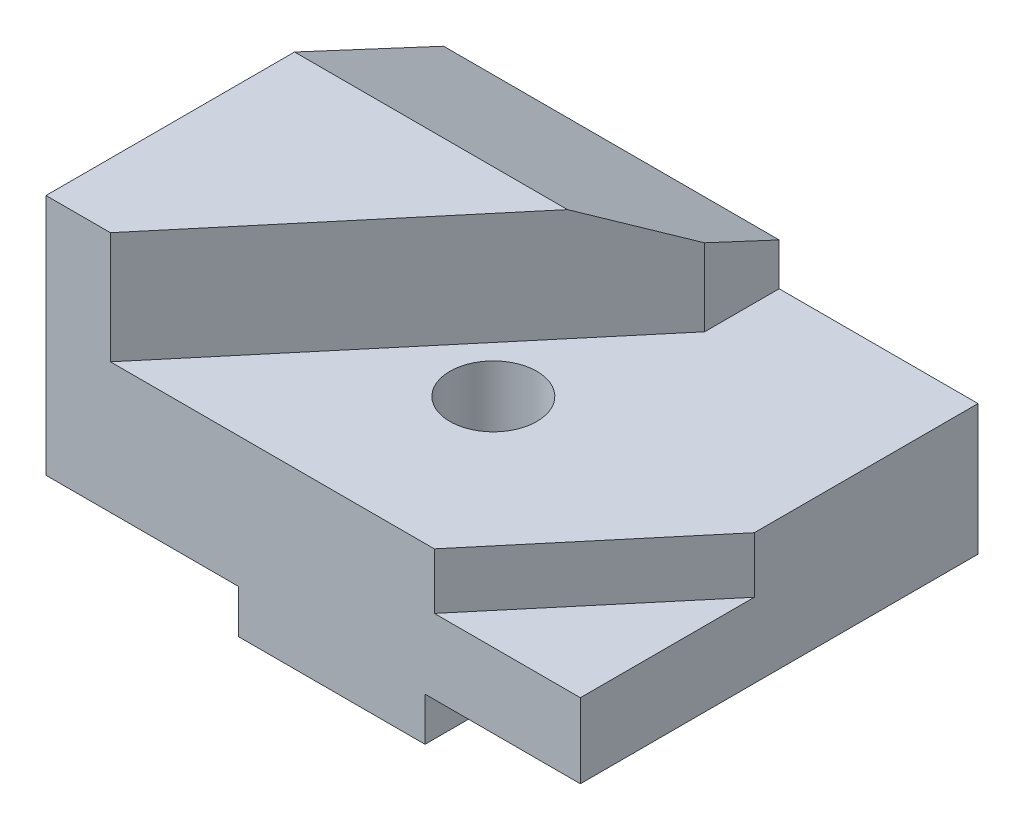
ISO-10303-21;
HEADER;
FILE_DESCRIPTION(('STEP AP214'),'2;1');
FILE_NAME('part.step','',(''),(''),'','','');
FILE_SCHEMA(('AUTOMOTIVE_DESIGN { 1 0 10303 214 1 1 1 1 }'));
ENDSEC;
DATA;
#1=APPLICATION_CONTEXT('core data for automotive mechanical design processes');
#2=APPLICATION_PROTOCOL_DEFINITION('international standard','automotive_design',2000,#1);
#3=PRODUCT_CONTEXT('',#1,'mechanical');
#4=PRODUCT('Part','Part','',(#3));
#5=PRODUCT_RELATED_PRODUCT_CATEGORY('part','',(#4));
#6=PRODUCT_DEFINITION_FORMATION('','',#4);
#7=PRODUCT_DEFINITION_CONTEXT('part definition',#1,'design');
#8=PRODUCT_DEFINITION('design','',#6,#7);
#9=PRODUCT_DEFINITION_SHAPE('','',#8);
#10=(LENGTH_UNIT() NAMED_UNIT(*) SI_UNIT(.MILLI.,.METRE.));
#11=(NAMED_UNIT(*) PLANE_ANGLE_UNIT() SI_UNIT($,.RADIAN.));
#12=(NAMED_UNIT(*) SI_UNIT($,.STERADIAN.) SOLID_ANGLE_UNIT());
#13=UNCERTAINTY_MEASURE_WITH_UNIT(LENGTH_MEASURE(1.E-05),#10,'distance_accuracy_value','');
#14=(GEOMETRIC_REPRESENTATION_CONTEXT(3) GLOBAL_UNCERTAINTY_ASSIGNED_CONTEXT((#13)) GLOBAL_UNIT_ASSIGNED_CONTEXT((#10,
#11,#12)) REPRESENTATION_CONTEXT('',''));
#15=CARTESIAN_POINT('',(0.,0.,0.));
#16=DIRECTION('',(0.,0.,1.));
#17=DIRECTION('',(1.,0.,0.));
#18=AXIS2_PLACEMENT_3D('',#15,#16,#17);
#19=CARTESIAN_POINT('',(0.,0.,0.));
#20=DIRECTION('',(0.,-1.,0.));
#21=DIRECTION('',(0.,0.,-1.));
#22=AXIS2_PLACEMENT_3D('',#19,#20,#21);
#23=PLANE('',#22);
#24=DIRECTION('',(-1.,0.,0.));
#25=VECTOR('',#24,1.);
#26=CARTESIAN_POINT('',(-43.,0.,-32.));
#27=LINE('',#26,#25);
#28=CARTESIAN_POINT('',(-12.,0.,-32.));
#29=VERTEX_POINT('',#28);
#30=CARTESIAN_POINT('',(-43.,0.,-32.));
#31=VERTEX_POINT('',#30);
#32=EDGE_CURVE('E231',#29,#31,#27,.T.);
#33=ORIENTED_EDGE('',*,*,#32,.F.);
#34=DIRECTION('',(0.,0.,1.));
#35=VECTOR('',#34,1.);
#36=CARTESIAN_POINT('',(-12.,0.,-32.));
#37=LINE('',#36,#35);
#38=CARTESIAN_POINT('',(-12.,0.,32.));
#39=VERTEX_POINT('',#38);
#40=EDGE_CURVE('E157',#29,#39,#37,.T.);
#41=ORIENTED_EDGE('',*,*,#40,.T.);
#42=DIRECTION('',(1.,0.,0.));
#43=VECTOR('',#42,1.);
#44=CARTESIAN_POINT('',(-43.,0.,32.));
#45=LINE('',#44,#43);
#46=CARTESIAN_POINT('',(-43.,0.,32.));
#47=VERTEX_POINT('',#46);
#48=EDGE_CURVE('E227',#47,#39,#45,.T.);
#49=ORIENTED_EDGE('',*,*,#48,.F.);
#50=DIRECTION('',(0.,0.,1.));
#51=VECTOR('',#50,1.);
#52=CARTESIAN_POINT('',(-43.,0.,32.));
#53=LINE('',#52,#51);
#54=EDGE_CURVE('E236',#31,#47,#53,.T.);
#55=ORIENTED_EDGE('',*,*,#54,.F.);
#56=EDGE_LOOP('',(#33,#41,#49,#55));
#57=FACE_BOUND('',#56,.T.);
#58=ADVANCED_FACE('F39',(#57),#23,.T.);
#59=CARTESIAN_POINT('',(43.,39.,32.));
#60=DIRECTION('',(-1.,0.,0.));
#61=DIRECTION('',(0.,0.,1.));
#62=AXIS2_PLACEMENT_3D('',#59,#60,#61);
#63=PLANE('',#62);
#64=DIRECTION('',(0.,0.,-1.));
#65=VECTOR('',#64,1.);
#66=CARTESIAN_POINT('',(43.,21.,-32.));
#67=LINE('',#66,#65);
#68=CARTESIAN_POINT('',(43.,21.,3.99697111651239));
#69=VERTEX_POINT('',#68);
#70=CARTESIAN_POINT('',(43.,21.,-32.));
#71=VERTEX_POINT('',#70);
#72=EDGE_CURVE('E206',#69,#71,#67,.T.);
#73=ORIENTED_EDGE('',*,*,#72,.F.);
#74=DIRECTION('',(0.,1.,0.));
#75=VECTOR('',#74,1.);
#76=CARTESIAN_POINT('',(43.,12.,3.99697111651239));
#77=LINE('',#76,#75);
#78=CARTESIAN_POINT('',(43.,12.,3.99697111651239));
#79=VERTEX_POINT('',#78);
#80=EDGE_CURVE('E190',#79,#69,#77,.T.);
#81=ORIENTED_EDGE('',*,*,#80,.F.);
#82=DIRECTION('',(0.,0.,-1.));
#83=VECTOR('',#82,1.);
#84=CARTESIAN_POINT('',(43.,12.,32.));
#85=LINE('',#84,#83);
#86=CARTESIAN_POINT('',(43.,12.,32.));
#87=VERTEX_POINT('',#86);
#88=EDGE_CURVE('E180',#87,#79,#85,.T.);
#89=ORIENTED_EDGE('',*,*,#88,.F.);
#90=DIRECTION('',(0.,-1.,0.));
#91=VECTOR('',#90,1.);
#92=CARTESIAN_POINT('',(43.,39.,32.));
#93=LINE('',#92,#91);
#94=CARTESIAN_POINT('',(43.,0.,32.));
#95=VERTEX_POINT('',#94);
#96=EDGE_CURVE('E229',#87,#95,#93,.T.);
#97=ORIENTED_EDGE('',*,*,#96,.T.);
#98=DIRECTION('',(0.,0.,-1.));
#99=VECTOR('',#98,1.);
#100=CARTESIAN_POINT('',(43.,0.,32.));
#101=LINE('',#100,#99);
#102=CARTESIAN_POINT('',(43.,0.,-32.));
#103=VERTEX_POINT('',#102);
#104=EDGE_CURVE('E225',#95,#103,#101,.T.);
#105=ORIENTED_EDGE('',*,*,#104,.T.);
#106=DIRECTION('',(0.,-1.,0.));
#107=VECTOR('',#106,1.);
#108=CARTESIAN_POINT('',(43.,39.,-32.));
#109=LINE('',#108,#107);
#110=EDGE_CURVE('E248',#71,#103,#109,.T.);
#111=ORIENTED_EDGE('',*,*,#110,.F.);
#112=EDGE_LOOP('',(#73,#81,#89,#97,#105,#111));
#113=FACE_BOUND('',#112,.T.);
#114=ADVANCED_FACE('F41',(#113),#63,.F.);
#115=CARTESIAN_POINT('',(-43.,39.,-32.));
#116=DIRECTION('',(0.,0.,1.));
#117=DIRECTION('',(1.,0.,0.));
#118=AXIS2_PLACEMENT_3D('',#115,#116,#117);
#119=PLANE('',#118);
#120=DIRECTION('',(1.,0.,0.));
#121=VECTOR('',#120,1.);
#122=CARTESIAN_POINT('',(-86.,27.80861620428,-32.));
#123=LINE('',#122,#121);
#124=CARTESIAN_POINT('',(-43.,27.80861620428,-32.));
#125=VERTEX_POINT('',#124);
#126=CARTESIAN_POINT('',(11.,27.80861620428,-32.));
#127=VERTEX_POINT('',#126);
#128=EDGE_CURVE('E211',#125,#127,#123,.T.);
#129=ORIENTED_EDGE('',*,*,#128,.T.);
#130=DIRECTION('',(0.,1.,0.));
#131=VECTOR('',#130,1.);
#132=CARTESIAN_POINT('',(11.,21.,-32.));
#133=LINE('',#132,#131);
#134=CARTESIAN_POINT('',(11.,21.,-32.));
#135=VERTEX_POINT('',#134);
#136=EDGE_CURVE('E65',#135,#127,#133,.T.);
#137=ORIENTED_EDGE('',*,*,#136,.F.);
#138=DIRECTION('',(-1.,0.,0.));
#139=VECTOR('',#138,1.);
#140=CARTESIAN_POINT('',(11.,21.,-32.));
#141=LINE('',#140,#139);
#142=EDGE_CURVE('E194',#71,#135,#141,.T.);
#143=ORIENTED_EDGE('',*,*,#142,.F.);
#144=ORIENTED_EDGE('',*,*,#110,.T.);
#145=CARTESIAN_POINT('',(18.,0.,-32.));
#146=VERTEX_POINT('',#145);
#147=EDGE_CURVE('E234',#103,#146,#27,.T.);
#148=ORIENTED_EDGE('',*,*,#147,.T.);
#149=DIRECTION('',(0.,1.,0.));
#150=VECTOR('',#149,1.);
#151=CARTESIAN_POINT('',(18.,0.,-32.));
#152=LINE('',#151,#150);
#153=CARTESIAN_POINT('',(18.,-7.,-32.));
#154=VERTEX_POINT('',#153);
#155=EDGE_CURVE('E149',#154,#146,#152,.T.);
#156=ORIENTED_EDGE('',*,*,#155,.F.);
#157=DIRECTION('',(1.,0.,0.));
#158=VECTOR('',#157,1.);
#159=CARTESIAN_POINT('',(-12.,-7.,-32.));
#160=LINE('',#159,#158);
#161=CARTESIAN_POINT('',(-12.,-7.,-32.));
#162=VERTEX_POINT('',#161);
#163=EDGE_CURVE('E141',#162,#154,#160,.T.);
#164=ORIENTED_EDGE('',*,*,#163,.F.);
#165=DIRECTION('',(0.,-1.,0.));
#166=VECTOR('',#165,1.);
#167=CARTESIAN_POINT('',(-12.,0.,-32.));
#168=LINE('',#167,#166);
#169=EDGE_CURVE('E152',#29,#162,#168,.T.);
#170=ORIENTED_EDGE('',*,*,#169,.F.);
#171=ORIENTED_EDGE('',*,*,#32,.T.);
#172=DIRECTION('',(0.,-1.,0.));
#173=VECTOR('',#172,1.);
#174=CARTESIAN_POINT('',(-43.,39.,-32.));
#175=LINE('',#174,#173);
#176=EDGE_CURVE('E246',#125,#31,#175,.T.);
#177=ORIENTED_EDGE('',*,*,#176,.F.);
#178=EDGE_LOOP('',(#129,#137,#143,#144,#148,#156,#164,#170,#171,#177));
#179=FACE_BOUND('',#178,.T.);
#180=ADVANCED_FACE('F153',(#179),#119,.F.);
#181=CARTESIAN_POINT('',(-43.,39.,32.));
#182=DIRECTION('',(1.,0.,0.));
#183=DIRECTION('',(0.,0.,-1.));
#184=AXIS2_PLACEMENT_3D('',#181,#182,#183);
#185=PLANE('',#184);
#186=DIRECTION('',(0.,0.,1.));
#187=VECTOR('',#186,1.);
#188=CARTESIAN_POINT('',(-43.,39.,32.));
#189=LINE('',#188,#187);
#190=CARTESIAN_POINT('',(-43.,39.,-8.));
#191=VERTEX_POINT('',#190);
#192=CARTESIAN_POINT('',(-43.,39.,32.));
#193=VERTEX_POINT('',#192);
#194=EDGE_CURVE('E223',#191,#193,#189,.T.);
#195=ORIENTED_EDGE('',*,*,#194,.F.);
#196=DIRECTION('',(0.,-0.4226182617407,-0.90630778703665));
#197=VECTOR('',#196,1.);
#198=CARTESIAN_POINT('',(-43.,54.3208888623796,24.8557521937308));
#199=LINE('',#198,#197);
#200=EDGE_CURVE('E217',#191,#125,#199,.T.);
#201=ORIENTED_EDGE('',*,*,#200,.T.);
#202=ORIENTED_EDGE('',*,*,#176,.T.);
#203=ORIENTED_EDGE('',*,*,#54,.T.);
#204=DIRECTION('',(0.,-1.,0.));
#205=VECTOR('',#204,1.);
#206=CARTESIAN_POINT('',(-43.,39.,32.));
#207=LINE('',#206,#205);
#208=EDGE_CURVE('E243',#193,#47,#207,.T.);
#209=ORIENTED_EDGE('',*,*,#208,.F.);
#210=EDGE_LOOP('',(#195,#201,#202,#203,#209));
#211=FACE_BOUND('',#210,.T.);
#212=ADVANCED_FACE('F264',(#211),#185,.F.);
#213=CARTESIAN_POINT('',(-43.,39.,32.));
#214=DIRECTION('',(0.,0.,-1.));
#215=DIRECTION('',(-1.,0.,0.));
#216=AXIS2_PLACEMENT_3D('',#213,#214,#215);
#217=PLANE('',#216);
#218=DIRECTION('',(1.,0.,0.));
#219=VECTOR('',#218,1.);
#220=CARTESIAN_POINT('',(19.5026687920191,12.,32.));
#221=LINE('',#220,#219);
#222=CARTESIAN_POINT('',(19.5026687920191,12.,32.));
#223=VERTEX_POINT('',#222);
#224=EDGE_CURVE('E184',#223,#87,#221,.T.);
#225=ORIENTED_EDGE('',*,*,#224,.F.);
#226=DIRECTION('',(0.,1.,0.));
#227=VECTOR('',#226,1.);
#228=CARTESIAN_POINT('',(19.5026687920191,12.,32.));
#229=LINE('',#228,#227);
#230=CARTESIAN_POINT('',(19.5026687920191,21.,32.));
#231=VERTEX_POINT('',#230);
#232=EDGE_CURVE('E189',#223,#231,#229,.T.);
#233=ORIENTED_EDGE('',*,*,#232,.T.);
#234=DIRECTION('',(1.,0.,0.));
#235=VECTOR('',#234,1.);
#236=CARTESIAN_POINT('',(-32.633180821218,21.,32.));
#237=LINE('',#236,#235);
#238=CARTESIAN_POINT('',(-32.633180821218,21.,32.));
#239=VERTEX_POINT('',#238);
#240=EDGE_CURVE('E201',#239,#231,#237,.T.);
#241=ORIENTED_EDGE('',*,*,#240,.F.);
#242=DIRECTION('',(0.,1.,0.));
#243=VECTOR('',#242,1.);
#244=CARTESIAN_POINT('',(-32.633180821218,21.,32.));
#245=LINE('',#244,#243);
#246=CARTESIAN_POINT('',(-32.633180821218,39.,32.));
#247=VERTEX_POINT('',#246);
#248=EDGE_CURVE('E212',#239,#247,#245,.T.);
#249=ORIENTED_EDGE('',*,*,#248,.T.);
#250=DIRECTION('',(1.,0.,0.));
#251=VECTOR('',#250,1.);
#252=CARTESIAN_POINT('',(-43.,39.,32.));
#253=LINE('',#252,#251);
#254=EDGE_CURVE('E228',#193,#247,#253,.T.);
#255=ORIENTED_EDGE('',*,*,#254,.F.);
#256=ORIENTED_EDGE('',*,*,#208,.T.);
#257=ORIENTED_EDGE('',*,*,#48,.T.);
#258=DIRECTION('',(0.,-1.,0.));
#259=VECTOR('',#258,1.);
#260=CARTESIAN_POINT('',(-12.,0.,32.));
#261=LINE('',#260,#259);
#262=CARTESIAN_POINT('',(-12.,-7.,32.));
#263=VERTEX_POINT('',#262);
#264=EDGE_CURVE('E53',#39,#263,#261,.T.);
#265=ORIENTED_EDGE('',*,*,#264,.T.);
#266=DIRECTION('',(1.,0.,0.));
#267=VECTOR('',#266,1.);
#268=CARTESIAN_POINT('',(-12.,-7.,32.));
#269=LINE('',#268,#267);
#270=CARTESIAN_POINT('',(18.,-7.,32.));
#271=VERTEX_POINT('',#270);
#272=EDGE_CURVE('E143',#263,#271,#269,.T.);
#273=ORIENTED_EDGE('',*,*,#272,.T.);
#274=DIRECTION('',(0.,1.,0.));
#275=VECTOR('',#274,1.);
#276=CARTESIAN_POINT('',(18.,0.,32.));
#277=LINE('',#276,#275);
#278=CARTESIAN_POINT('',(18.,0.,32.));
#279=VERTEX_POINT('',#278);
#280=EDGE_CURVE('E163',#271,#279,#277,.T.);
#281=ORIENTED_EDGE('',*,*,#280,.T.);
#282=EDGE_CURVE('E238',#279,#95,#45,.T.);
#283=ORIENTED_EDGE('',*,*,#282,.T.);
#284=ORIENTED_EDGE('',*,*,#96,.F.);
#285=EDGE_LOOP('',(#225,#233,#241,#249,#255,#256,#257,#265,#273,#281,#283,#284));
#286=FACE_BOUND('',#285,.T.);
#287=ADVANCED_FACE('F266',(#286),#217,.F.);
#288=CARTESIAN_POINT('',(0.,39.,0.));
#289=DIRECTION('',(0.,-1.,0.));
#290=DIRECTION('',(0.,0.,-1.));
#291=AXIS2_PLACEMENT_3D('',#288,#289,#290);
#292=PLANE('',#291);
#293=ORIENTED_EDGE('',*,*,#254,.T.);
#294=DIRECTION('',(-0.642787609686535,0.,0.766044443118982));
#295=VECTOR('',#294,1.);
#296=CARTESIAN_POINT('',(11.,39.,-20.));
#297=LINE('',#296,#295);
#298=CARTESIAN_POINT('',(0.93080442587276,39.,-8.));
#299=VERTEX_POINT('',#298);
#300=EDGE_CURVE('E192',#299,#247,#297,.T.);
#301=ORIENTED_EDGE('',*,*,#300,.F.);
#302=DIRECTION('',(-1.,0.,0.));
#303=VECTOR('',#302,1.);
#304=CARTESIAN_POINT('',(0.,39.,-8.));
#305=LINE('',#304,#303);
#306=EDGE_CURVE('E252',#299,#191,#305,.T.);
#307=ORIENTED_EDGE('',*,*,#306,.T.);
#308=ORIENTED_EDGE('',*,*,#194,.T.);
#309=EDGE_LOOP('',(#293,#301,#307,#308));
#310=FACE_BOUND('',#309,.T.);
#311=ADVANCED_FACE('F267',(#310),#292,.F.);
#312=DIRECTION('',(0.,0.,1.));
#313=VECTOR('',#312,1.);
#314=CARTESIAN_POINT('',(18.,0.,-32.));
#315=LINE('',#314,#313);
#316=EDGE_CURVE('E171',#146,#279,#315,.T.);
#317=ORIENTED_EDGE('',*,*,#316,.F.);
#318=ORIENTED_EDGE('',*,*,#147,.F.);
#319=ORIENTED_EDGE('',*,*,#104,.F.);
#320=ORIENTED_EDGE('',*,*,#282,.F.);
#321=EDGE_LOOP('',(#317,#318,#319,#320));
#322=FACE_BOUND('',#321,.T.);
#323=ADVANCED_FACE('F287',(#322),#23,.T.);
#324=CARTESIAN_POINT('',(-86.,39.,-8.));
#325=DIRECTION('',(0.,-0.90630778703665,0.4226182617407));
#326=DIRECTION('',(0.,-0.4226182617407,-0.90630778703665));
#327=AXIS2_PLACEMENT_3D('',#324,#325,#326);
#328=PLANE('',#327);
#329=ORIENTED_EDGE('',*,*,#306,.F.);
#330=DIRECTION('',(0.605326699380337,-0.336394469880428,-0.721400268679721));
#331=VECTOR('',#330,1.);
#332=CARTESIAN_POINT('',(-30.9224168327732,56.7015940156864,29.9611908706901));
#333=LINE('',#332,#331);
#334=CARTESIAN_POINT('',(11.,33.40430810214,-20.));
#335=VERTEX_POINT('',#334);
#336=EDGE_CURVE('E11',#299,#335,#333,.T.);
#337=ORIENTED_EDGE('',*,*,#336,.T.);
#338=DIRECTION('',(0.,-0.4226182617407,-0.90630778703665));
#339=VECTOR('',#338,1.);
#340=CARTESIAN_POINT('',(11.,39.,-8.));
#341=LINE('',#340,#339);
#342=EDGE_CURVE('E50',#335,#127,#341,.T.);
#343=ORIENTED_EDGE('',*,*,#342,.T.);
#344=ORIENTED_EDGE('',*,*,#128,.F.);
#345=ORIENTED_EDGE('',*,*,#200,.F.);
#346=EDGE_LOOP('',(#329,#337,#343,#344,#345));
#347=FACE_BOUND('',#346,.T.);
#348=ADVANCED_FACE('F251',(#347),#328,.F.);
#349=CARTESIAN_POINT('',(11.,21.,-20.));
#350=DIRECTION('',(-0.766044443118982,0.,-0.642787609686535));
#351=DIRECTION('',(-0.642787609686535,0.,0.766044443118982));
#352=AXIS2_PLACEMENT_3D('',#349,#350,#351);
#353=PLANE('',#352);
#354=ORIENTED_EDGE('',*,*,#300,.T.);
#355=ORIENTED_EDGE('',*,*,#248,.F.);
#356=DIRECTION('',(-0.642787609686535,0.,0.766044443118982));
#357=VECTOR('',#356,1.);
#358=CARTESIAN_POINT('',(11.,21.,-20.));
#359=LINE('',#358,#357);
#360=CARTESIAN_POINT('',(11.,21.,-20.));
#361=VERTEX_POINT('',#360);
#362=EDGE_CURVE('E198',#361,#239,#359,.T.);
#363=ORIENTED_EDGE('',*,*,#362,.F.);
#364=DIRECTION('',(0.,1.,0.));
#365=VECTOR('',#364,1.);
#366=CARTESIAN_POINT('',(11.,21.,-20.));
#367=LINE('',#366,#365);
#368=EDGE_CURVE('E213',#361,#335,#367,.T.);
#369=ORIENTED_EDGE('',*,*,#368,.T.);
#370=ORIENTED_EDGE('',*,*,#336,.F.);
#371=EDGE_LOOP('',(#354,#355,#363,#369,#370));
#372=FACE_BOUND('',#371,.T.);
#373=ADVANCED_FACE('F271',(#372),#353,.F.);
#374=CARTESIAN_POINT('',(11.,21.,-32.));
#375=DIRECTION('',(-1.,0.,0.));
#376=DIRECTION('',(0.,0.,1.));
#377=AXIS2_PLACEMENT_3D('',#374,#375,#376);
#378=PLANE('',#377);
#379=ORIENTED_EDGE('',*,*,#368,.F.);
#380=DIRECTION('',(0.,0.,1.));
#381=VECTOR('',#380,1.);
#382=CARTESIAN_POINT('',(11.,21.,-32.));
#383=LINE('',#382,#381);
#384=EDGE_CURVE('E199',#135,#361,#383,.T.);
#385=ORIENTED_EDGE('',*,*,#384,.F.);
#386=ORIENTED_EDGE('',*,*,#136,.T.);
#387=ORIENTED_EDGE('',*,*,#342,.F.);
#388=EDGE_LOOP('',(#379,#385,#386,#387));
#389=FACE_BOUND('',#388,.T.);
#390=ADVANCED_FACE('F276',(#389),#378,.F.);
#391=CARTESIAN_POINT('',(0.,21.,0.));
#392=DIRECTION('',(0.,-1.,0.));
#393=DIRECTION('',(0.,0.,-1.));
#394=AXIS2_PLACEMENT_3D('',#391,#392,#393);
#395=PLANE('',#394);
#396=CARTESIAN_POINT('',(3.00000000000001,21.,6.));
#397=DIRECTION('',(0.,-1.,0.));
#398=DIRECTION('',(0.,0.,-1.));
#399=AXIS2_PLACEMENT_3D('',#396,#397,#398);
#400=CIRCLE('',#399,7.);
#401=CARTESIAN_POINT('',(3.00000000000001,21.,-0.999999999999998));
#402=VERTEX_POINT('',#401);
#403=EDGE_CURVE('E172',#402,#402,#400,.T.);
#404=ORIENTED_EDGE('',*,*,#403,.T.);
#405=EDGE_LOOP('',(#404));
#406=FACE_BOUND('',#405,.T.);
#407=ORIENTED_EDGE('',*,*,#142,.T.);
#408=ORIENTED_EDGE('',*,*,#384,.T.);
#409=ORIENTED_EDGE('',*,*,#362,.T.);
#410=ORIENTED_EDGE('',*,*,#240,.T.);
#411=DIRECTION('',(0.642787609686535,0.,-0.766044443118982));
#412=VECTOR('',#411,1.);
#413=CARTESIAN_POINT('',(19.5026687920191,21.,32.));
#414=LINE('',#413,#412);
#415=EDGE_CURVE('E202',#231,#69,#414,.T.);
#416=ORIENTED_EDGE('',*,*,#415,.T.);
#417=ORIENTED_EDGE('',*,*,#72,.T.);
#418=EDGE_LOOP('',(#407,#408,#409,#410,#416,#417));
#419=FACE_BOUND('',#418,.T.);
#420=ADVANCED_FACE('F280',(#406,#419),#395,.F.);
#421=CARTESIAN_POINT('',(43.,12.,3.99697111651239));
#422=DIRECTION('',(-0.766044443118982,0.,-0.642787609686535));
#423=DIRECTION('',(-0.642787609686535,0.,0.766044443118982));
#424=AXIS2_PLACEMENT_3D('',#421,#422,#423);
#425=PLANE('',#424);
#426=ORIENTED_EDGE('',*,*,#232,.F.);
#427=DIRECTION('',(-0.642787609686535,0.,0.766044443118982));
#428=VECTOR('',#427,1.);
#429=CARTESIAN_POINT('',(43.,12.,3.99697111651239));
#430=LINE('',#429,#428);
#431=EDGE_CURVE('E185',#79,#223,#430,.T.);
#432=ORIENTED_EDGE('',*,*,#431,.F.);
#433=ORIENTED_EDGE('',*,*,#80,.T.);
#434=ORIENTED_EDGE('',*,*,#415,.F.);
#435=EDGE_LOOP('',(#426,#432,#433,#434));
#436=FACE_BOUND('',#435,.T.);
#437=ADVANCED_FACE('F300',(#436),#425,.F.);
#438=CARTESIAN_POINT('',(0.,12.,0.));
#439=DIRECTION('',(0.,-1.,0.));
#440=DIRECTION('',(0.,0.,-1.));
#441=AXIS2_PLACEMENT_3D('',#438,#439,#440);
#442=PLANE('',#441);
#443=ORIENTED_EDGE('',*,*,#88,.T.);
#444=ORIENTED_EDGE('',*,*,#431,.T.);
#445=ORIENTED_EDGE('',*,*,#224,.T.);
#446=EDGE_LOOP('',(#443,#444,#445));
#447=FACE_BOUND('',#446,.T.);
#448=ADVANCED_FACE('F294',(#447),#442,.F.);
#449=CARTESIAN_POINT('',(3.00000000000001,-58.,6.));
#450=DIRECTION('',(0.,1.,0.));
#451=DIRECTION('',(0.,0.,1.));
#452=AXIS2_PLACEMENT_3D('',#449,#450,#451);
#453=CYLINDRICAL_SURFACE('',#452,7.);
#454=CARTESIAN_POINT('',(3.00000000000001,0.,6.));
#455=DIRECTION('',(0.,-1.,0.));
#456=DIRECTION('',(0.,0.,-1.));
#457=AXIS2_PLACEMENT_3D('',#454,#455,#456);
#458=CIRCLE('',#457,7.);
#459=CARTESIAN_POINT('',(3.00000000000001,0.,-0.999999999999998));
#460=VERTEX_POINT('',#459);
#461=EDGE_CURVE('E167',#460,#460,#458,.T.);
#462=ORIENTED_EDGE('',*,*,#461,.T.);
#463=EDGE_LOOP('',(#462));
#464=FACE_BOUND('',#463,.T.);
#465=ORIENTED_EDGE('',*,*,#403,.F.);
#466=EDGE_LOOP('',(#465));
#467=FACE_BOUND('',#466,.T.);
#468=ADVANCED_FACE('F302',(#464,#467),#453,.F.);
#469=CARTESIAN_POINT('',(-12.,-7.,-32.));
#470=DIRECTION('',(0.,-1.,0.));
#471=DIRECTION('',(0.,0.,-1.));
#472=AXIS2_PLACEMENT_3D('',#469,#470,#471);
#473=PLANE('',#472);
#474=ORIENTED_EDGE('',*,*,#272,.F.);
#475=DIRECTION('',(0.,0.,1.));
#476=VECTOR('',#475,1.);
#477=CARTESIAN_POINT('',(-12.,-7.,-32.));
#478=LINE('',#477,#476);
#479=EDGE_CURVE('E137',#162,#263,#478,.T.);
#480=ORIENTED_EDGE('',*,*,#479,.F.);
#481=ORIENTED_EDGE('',*,*,#163,.T.);
#482=DIRECTION('',(0.,0.,1.));
#483=VECTOR('',#482,1.);
#484=CARTESIAN_POINT('',(18.,-7.,-32.));
#485=LINE('',#484,#483);
#486=EDGE_CURVE('E150',#154,#271,#485,.T.);
#487=ORIENTED_EDGE('',*,*,#486,.T.);
#488=EDGE_LOOP('',(#474,#480,#481,#487));
#489=FACE_BOUND('',#488,.T.);
#490=ADVANCED_FACE('F145',(#489),#473,.T.);
#491=CARTESIAN_POINT('',(18.,0.,-32.));
#492=DIRECTION('',(1.,0.,0.));
#493=DIRECTION('',(0.,0.,-1.));
#494=AXIS2_PLACEMENT_3D('',#491,#492,#493);
#495=PLANE('',#494);
#496=ORIENTED_EDGE('',*,*,#280,.F.);
#497=ORIENTED_EDGE('',*,*,#486,.F.);
#498=ORIENTED_EDGE('',*,*,#155,.T.);
#499=ORIENTED_EDGE('',*,*,#316,.T.);
#500=EDGE_LOOP('',(#496,#497,#498,#499));
#501=FACE_BOUND('',#500,.T.);
#502=ADVANCED_FACE('F291',(#501),#495,.T.);
#503=CARTESIAN_POINT('',(-12.,0.,-32.));
#504=DIRECTION('',(-1.,0.,0.));
#505=DIRECTION('',(0.,0.,1.));
#506=AXIS2_PLACEMENT_3D('',#503,#504,#505);
#507=PLANE('',#506);
#508=ORIENTED_EDGE('',*,*,#264,.F.);
#509=ORIENTED_EDGE('',*,*,#40,.F.);
#510=ORIENTED_EDGE('',*,*,#169,.T.);
#511=ORIENTED_EDGE('',*,*,#479,.T.);
#512=EDGE_LOOP('',(#508,#509,#510,#511));
#513=FACE_BOUND('',#512,.T.);
#514=ADVANCED_FACE('F158',(#513),#507,.T.);
#515=CARTESIAN_POINT('',(-12.,0.,-32.));
#516=DIRECTION('',(0.,1.,0.));
#517=DIRECTION('',(0.,0.,1.));
#518=AXIS2_PLACEMENT_3D('',#515,#516,#517);
#519=PLANE('',#518);
#520=ORIENTED_EDGE('',*,*,#461,.F.);
#521=EDGE_LOOP('',(#520));
#522=FACE_BOUND('',#521,.T.);
#523=ADVANCED_FACE('F412',(#522),#519,.T.);
#524=CLOSED_SHELL('',(#58,#114,#180,#212,#287,#311,#323,#348,#373,#390,#420,#437,#448,#468,#490,
#502,#514,#523));
#525=MANIFOLD_SOLID_BREP('B2',#524);
#526=ADVANCED_BREP_SHAPE_REPRESENTATION('',(#18,#525),#14);
#527=SHAPE_DEFINITION_REPRESENTATION(#9,#526);
ENDSEC;
END-ISO-10303-21;
